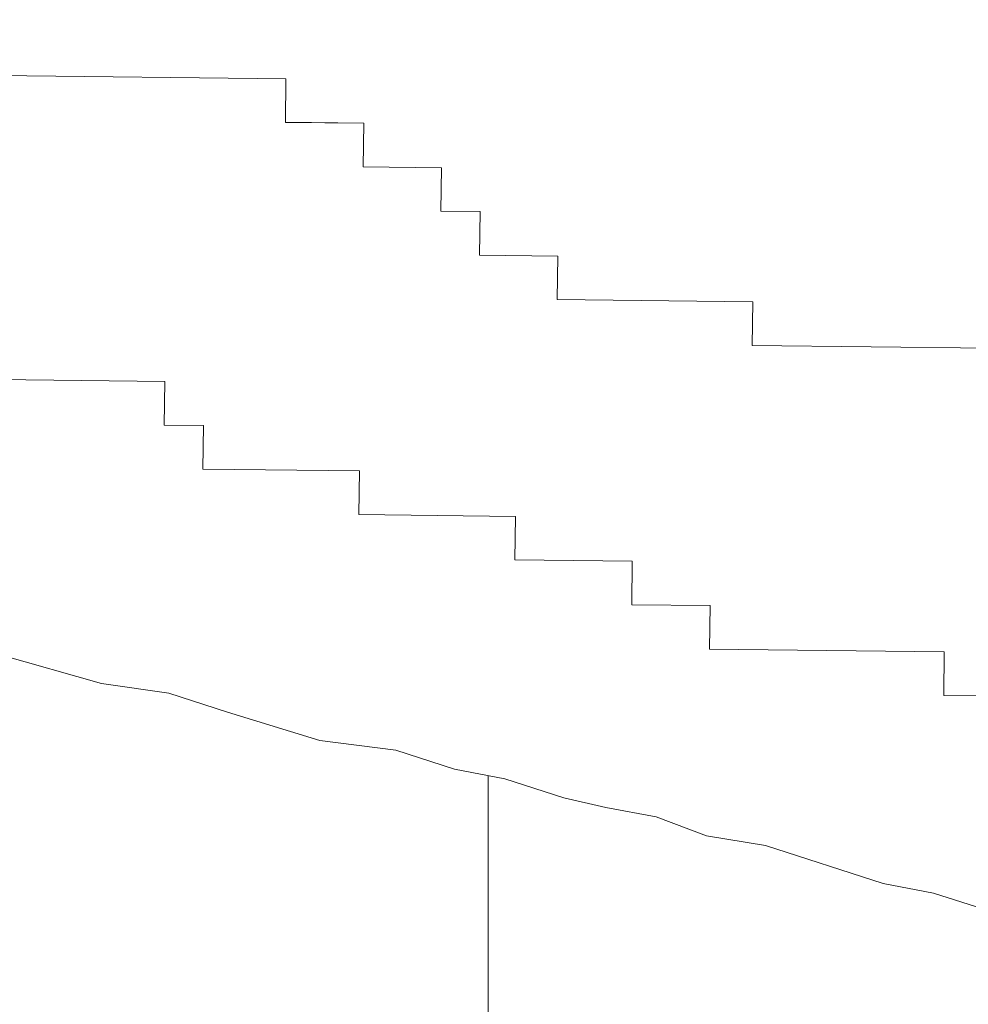
# Model space of a CAD drawing. Units: inches. Extents: x -466983 to 1020, y 324 to 318697.
# Tile 55 of 97: x 634.844 to 637.858, y 939.565 to 942.694. Entities that reach past the tile are written whole.
import ezdxf

# ---------------------------------------------------------------- set-up
doc = ezdxf.new("R2010")
doc.units = ezdxf.units.IN
doc.header["$MEASUREMENT"] = 0
doc.layers.add('A-FLOR-PATT', color=252, linetype='Continuous', lineweight=13)
doc.layers.add('A-FURN', color=8, linetype='Continuous', lineweight=18)

# ---------------------------------------------------------------- blocks, each defined once
blk = doc.blocks.new('L Shaped Sofa')
at = {"ltscale": 2}
for p, q in [((2432.347, 748.1215), (2432.347, 765.179)), ((2429.4248, 748.9121), (2429.7657, 748.8021)), ((2429.7657, 748.8021), (2430.0581, 748.7465)), ((2430.0581, 748.7465), (2430.74, 748.5264)), ((2430.74, 748.5264), (2431.0812, 748.4706)), ((2431.0812, 748.4706), (2431.3733, 748.3608)), ((2431.3733, 748.3608), (2431.6657, 748.3052)), ((2431.6657, 748.3052), (2431.9094, 748.2499)), ((2431.9094, 748.2499), (2432.2503, 748.1398)), ((2432.2503, 748.1398), (2432.5427, 748.0842)), ((2432.5427, 748.0842), (2432.8836, 747.9742)), ((2432.8836, 747.9742), (2433.3224, 747.9179)), ((2433.3224, 747.9179), (2433.8582, 747.7528)), ((2433.8582, 747.7528), (2434.1991, 747.6427)), ((2427.8919, 747.6787), (2429.7066, 747.6565)), ((2429.7066, 747.6565), (2429.7036, 747.4046)), ((2434.1991, 747.6427), (2434.5891, 747.5867)), ((2434.5891, 747.5867), (2435.1737, 747.4213)), ((2429.7036, 747.4046), (2431.0646, 747.388)), ((2431.0646, 747.388), (2431.0615, 747.1361)), ((2431.0615, 747.1361), (2431.5152, 747.1305)), ((2431.5152, 747.1305), (2431.5121, 746.8786)), ((2431.5121, 746.8786), (2432.1926, 746.8703)), ((2432.1926, 746.8703), (2432.1895, 746.6184)), ((2432.1895, 746.6184), (2433.0969, 746.6073)), ((2433.0969, 746.6073), (2433.0938, 746.3554)), ((2433.0938, 746.3554), (2434.0011, 746.3443)), ((2434.0011, 746.3443), (2433.9981, 746.0924)), ((2433.9981, 746.0924), (2434.2249, 746.0896)), ((2434.2249, 746.0896), (2434.2218, 745.8377)), ((2434.2218, 745.8377), (2436.2633, 745.8128)), ((2428.5478, 745.6551), (2430.8162, 745.6274)), ((2430.8162, 745.6274), (2430.8131, 745.3755)), ((2430.8131, 745.3755), (2431.9473, 745.3616)), ((2431.9473, 745.3616), (2431.9442, 745.1097)), ((2431.9442, 745.1097), (2432.3979, 745.1042)), ((2432.3979, 745.1042), (2432.3948, 744.8522)), ((2432.3948, 744.8522), (2432.6216, 744.8495)), ((2432.6216, 744.8495), (2432.6186, 744.5976)), ((2432.6186, 744.5976), (2433.0722, 744.592)), ((2433.0722, 744.592), (2433.0692, 744.3401)), ((2433.0692, 744.3401), (2433.5228, 744.3346)), ((2433.5228, 744.3346), (2433.5198, 744.0827)), ((2433.5198, 744.0827), (2436.015, 744.0522))]:
    blk.add_line(p, q, dxfattribs=at)

msp = doc.modelspace()

# ---------------------------------------------------------------- hatches: boundary and pattern name
at = {"layer": 'A-FLOR-PATT', "transparency": 33554572}
h = msp.add_hatch(dxfattribs=at)
h.set_pattern_fill('ANSI37', color=256, scale=30)
h.set_pattern_definition([(45, (-1212.4137, -290.035), (-2.6516504, 2.6516504), []), (135, (-1212.4137, -290.035), (-2.6516504, -2.6516504), [])])
h.paths.add_polyline_path([(901.8057, 1075.9377), (900.6144, 1075.9377), (900.6144, 1065.3856), (899.391, 1065.3856), (898.0911, 1065.3856), (892.8356, 1058.7098, -0.258377), (892.1875, 1058.3509), (879.9848, 1058.3509, -0.20177), (879.4382, 1058.5808), (874.0812, 1065.3856), (872.7813, 1065.3856), (871.5579, 1065.3856), (871.5579, 1075.9377), (813.8057, 1075.9377), (813.8057, 1044.7922), (832.3947, 1044.7922, -0.394795), (848.6602, 1028.5356), (848.6602, 1009.9377), (901.8057, 1009.9377), (901.8057, 1015.9377), (901.3057, 1015.9377), (871.3057, 1015.9377), (871.3057, 1017.2502), (871.3344, 1017.2502, -0.401453), (901.3057, 1045.9377), (901.8057, 1045.9377)])
edge = h.paths.add_edge_path(flags=16)
edge.add_line((847.7731, 1068.9486), (847.7731, 1073.7088))
edge.add_arc((849.2269, 1073.7088), 1.4538, 90, 180, ccw=False)
edge.add_line((849.2269, 1075.1627), (864.4921, 1075.1627))
edge.add_arc((864.4921, 1073.7088), 1.4538, 0, 90, ccw=False)
edge.add_line((865.9459, 1073.7088), (865.9459, 1069.0035))
edge.add_arc((832.6447, 1068.9761), 33.3012, -20.61234, 0.04725, ccw=False)
edge.add_ellipse((856.8595, 1058.48), major_axis=(0, 10.2131), ratio=0.6859192, start_angle=100.00884, end_angle=259.99116, ccw=False)
edge.add_arc((881.0742, 1068.9761), 33.3012, 180.04725, 200.61234, ccw=False)
h.paths.add_polyline_path([(853.1456, 1066.4815), (853.1456, 1066.4534), (853.1463, 1066.4534, 0.433107), (852.9166, 1066.6849), (852.9166, 1066.4534), (853.1456, 1066.4534), (853.1456, 1066.4815), (853.088, 1066.6122, 0.697939), (852.6995, 1066.4534), (852.7003, 1066.4534), (852.7003, 1066.4815), (852.9166, 1067.0012), (852.9166, 1066.6849, -0.396254)], flags=0)
h.paths.add_polyline_path([(861.0187, 1066.4815), (861.0187, 1066.4534), (861.0194, 1066.4534, 0.416404), (860.8024, 1066.6849), (860.8024, 1066.4534), (861.0187, 1066.4534), (861.0187, 1066.4815), (860.9672, 1066.6053, 0.713344), (860.5726, 1066.4534), (860.5734, 1066.4534), (860.5734, 1066.4815), (860.8024, 1067.0012), (860.8024, 1066.6849, -0.379973)], flags=0)
edge = h.paths.add_edge_path(flags=0)
edge.add_spline(control_points=[(861.1298, 1065.7855), (861.4661, 1065.2478), (861.6134, 1065.0161), (861.9833, 1064.3736), (862.1924, 1063.9443), (862.5614, 1063.0391), (862.7212, 1062.5633), (862.9865, 1061.5781), (863.092, 1061.0689), (863.2452, 1060.031), (863.293, 1059.5025), (863.3295, 1058.4409), (863.3181, 1057.9078), (863.2366, 1056.8518), (863.1664, 1056.3289), (862.9695, 1055.308), (862.8427, 1054.8099), (862.5365, 1053.8522), (862.3571, 1053.3927), (861.9514, 1052.5249), (861.7251, 1052.1166), (861.233, 1051.3622), (860.9672, 1051.0162), (860.4048, 1050.3949), (860.1082, 1050.1197), (859.4937, 1049.6461), (859.1758, 1049.4476), (858.5276, 1049.1299), (858.1973, 1049.0107), (857.5315, 1048.8518), (857.1959, 1048.8121), (856.5249, 1048.812), (856.1894, 1048.8515), (855.5236, 1049.0101), (855.1933, 1049.1291), (854.545, 1049.4465), (854.2271, 1049.6449), (853.6124, 1050.1183), (853.3158, 1050.3933), (852.7533, 1051.0143), (852.4874, 1051.3602), (851.9952, 1052.1144), (851.7688, 1052.5225), (851.3629, 1053.3902), (851.1834, 1053.8496), (850.877, 1054.8071), (850.7501, 1055.3051), (850.553, 1056.326), (850.4827, 1056.8488), (850.401, 1057.9048), (850.3895, 1058.4379), (850.4257, 1059.4995), (850.4734, 1060.0281), (850.6265, 1061.066), (850.7318, 1061.5753), (850.9969, 1062.5605), (851.1567, 1063.0365), (851.5254, 1063.9418), (851.7345, 1064.3712), (852.1056, 1065.0164), (852.2544, 1065.2503), (852.6082, 1065.7335)], knot_values=[3.915332, 3.915332, 3.915332, 3.915332, 4.013468, 4.013468, 4.175532, 4.175532, 4.337596, 4.337596, 4.49966, 4.49966, 4.661724, 4.661724, 4.823788, 4.823788, 4.985852, 4.985852, 5.147916, 5.147916, 5.30998, 5.30998, 5.472044, 5.472044, 5.634109, 5.634109, 5.796173, 5.796173, 5.958237, 5.958237, 6.120301, 6.120301, 6.282365, 6.282365, 6.444429, 6.444429, 6.606493, 6.606493, 6.768557, 6.768557, 6.930621, 6.930621, 7.092685, 7.092685, 7.254749, 7.254749, 7.416813, 7.416813, 7.578878, 7.578878, 7.740942, 7.740942, 7.903006, 7.903006, 8.06507, 8.06507, 8.227134, 8.227134, 8.389198, 8.389198, 8.551262, 8.551262, 8.65037, 8.65037, 8.65037, 8.65037], degree=3, periodic=0)
edge.add_line((852.6421, 1065.7855), (861.1298, 1065.7855))
edge = h.paths.add_edge_path(flags=0)
edge.add_ellipse((856.8496, 1057.7432), major_axis=(0, 7.7921), ratio=0.687861, start_angle=0, end_angle=360)
h.paths.add_polyline_path([(848.8634, 1069.3891), (848.8634, 1073.9605, -0.414214), (849.9538, 1075.0508), (863.7652, 1075.0508, -0.414214), (864.8555, 1073.9605), (864.8555, 1069.3891, -0.388936), (864.5237, 1069.027, -0.043561), (849.1953, 1069.027, -0.388936)], flags=0)
h.paths.add_polyline_path([(853.1006, 1068.1122, -1), (852.6775, 1068.1122, -1)], flags=0)
edge = h.paths.add_edge_path(flags=0)
edge.add_ellipse((856.8595, 1057.3378), major_axis=(0, 2.207), ratio=0.657164, start_angle=0, end_angle=360)
h.paths.add_polyline_path([(861.0415, 1068.1122, -1), (860.6184, 1068.1122, -1)], flags=0)
edge = h.paths.add_edge_path()
edge.add_line((573.9537, 1057.3412), (573.9537, 1075.9377))
edge.add_line((573.9537, 1075.9377), (558.7308, 1075.9377))
edge.add_line((558.7308, 1075.9377), (558.7308, 1065.3856))
edge.add_line((558.7308, 1065.3856), (557.5074, 1065.3856))
edge.add_line((557.5074, 1065.3856), (556.2075, 1065.3856))
edge.add_line((556.2075, 1065.3856), (550.952, 1058.7098))
edge.add_arc((550.3039, 1059.1155), 0.7646, 270, 327.9483, ccw=False)
edge.add_line((550.3039, 1058.3509), (538.1012, 1058.3509))
edge.add_arc((538.1012, 1059.1155), 0.7646, 224.3704, 270, ccw=False)
edge.add_line((537.5546, 1058.5808), (532.1976, 1065.3856))
edge.add_line((532.1976, 1065.3856), (530.8977, 1065.3856))
edge.add_line((530.8977, 1065.3856), (529.6743, 1065.3856))
edge.add_line((529.6743, 1065.3856), (529.6743, 1075.9377))
edge.add_line((529.6743, 1075.9377), (520.8057, 1075.9377))
edge.add_line((520.8057, 1075.9377), (520.8057, 1045.9377))
edge.add_line((520.8057, 1045.9377), (521.3057, 1045.9377))
edge.add_arc((521.3057, 1015.9377), 30, 2.50749, 90, ccw=False)
edge.add_line((551.277, 1017.2502), (551.3057, 1017.2502))
edge.add_line((551.3057, 1017.2502), (551.3057, 1015.9377))
edge.add_line((551.3057, 1015.9377), (520.8057, 1015.9377))
edge.add_line((520.8057, 1015.9377), (520.8057, 1009.9377))
edge.add_line((520.8057, 1009.9377), (559.1913, 1010.4022))
edge.add_arc((559.1913, 1011.856), 1.4538, 180, 270, ccw=False)
edge.add_line((557.7375, 1011.856), (557.7375, 1016.5613))
edge.add_arc((591.0386, 1016.5888), 33.3012, 159.38766, 180.04725, ccw=False)
edge.add_ellipse((566.8239, 1027.0848), major_axis=(0, 10.2131), ratio=0.6859192, start_angle=280.00884, end_angle=439.99116, ccw=False)
edge.add_arc((542.6091, 1016.5888), 33.3012, 0.04725, 20.61234, ccw=False)
edge.add_line((575.9103, 1016.6162), (575.9103, 1011.856))
edge.add_arc((574.4565, 1011.856), 1.4538, -90, 0, ccw=False)
edge.add_line((574.4565, 1010.4022), (608.8057, 1009.9377))
edge.add_line((608.8057, 1009.9377), (608.8057, 1041.0857))
edge.add_line((608.8057, 1041.0857), (590.2179, 1041.0857))
edge.add_arc((590.775, 1057.9074), 16.8309, 181.92775, 268.10321, ccw=False)
edge = h.paths.add_edge_path()
edge.add_ellipse((494.2443, 583.6204), major_axis=(0, 10.2131), ratio=0.6859192, start_angle=280.00884, end_angle=439.99116, ccw=False)
edge.add_arc((470.0296, 573.1243), 33.3012, 0.04725, 20.61234, ccw=False)
edge.add_line((503.3307, 573.1518), (503.3307, 568.3916))
edge.add_arc((501.8769, 568.3916), 1.4538, -90, 0, ccw=False)
edge.add_line((501.8769, 566.9377), (539.8057, 566.9377))
edge.add_line((539.8057, 566.9377), (539.8057, 572.9377))
edge.add_line((539.8057, 572.9377), (539.3057, 572.9377))
edge.add_line((539.3057, 572.9377), (509.3057, 572.9377))
edge.add_line((509.3057, 572.9377), (509.3057, 574.2502))
edge.add_line((509.3057, 574.2502), (509.3344, 574.2502))
edge.add_arc((539.3057, 572.9377), 30, 90, 177.49251, ccw=False)
edge.add_line((539.3057, 602.9377), (539.8057, 602.9377))
edge.add_line((539.8057, 602.9377), (539.8057, 626.9377))
edge.add_line((539.8057, 626.9377), (531.7718, 626.9377))
edge.add_line((531.7718, 626.9377), (531.7718, 616.3856))
edge.add_line((531.7718, 616.3856), (530.5484, 616.3856))
edge.add_line((530.5484, 616.3856), (529.2485, 616.3856))
edge.add_line((529.2485, 616.3856), (523.7105, 609.3509))
edge.add_line((523.7105, 609.3509), (510.7766, 609.3509))
edge.add_line((510.7766, 609.3509), (505.2386, 616.3856))
edge.add_line((505.2386, 616.3856), (503.9387, 616.3856))
edge.add_line((503.9387, 616.3856), (502.7153, 616.3856))
edge.add_line((502.7153, 616.3856), (502.7153, 626.9377))
edge.add_line((502.7153, 626.9377), (481.6983, 626.9377))
edge.add_line((481.6983, 626.9377), (481.6983, 610.995))
edge.add_arc((467.2703, 611.4728), 14.4359, 271.92775, 358.10321, ccw=False)
edge.add_line((467.7559, 597.0451), (451.8057, 597.0451))
edge.add_line((451.8057, 597.0451), (451.8057, 584.4035))
edge.add_line((451.8057, 584.4035), (451.8057, 566.9377))
edge.add_line((451.8057, 566.9377), (486.6117, 566.9377))
edge.add_arc((486.6117, 568.3916), 1.4538, 180, 270, ccw=False)
edge.add_line((485.1579, 568.3916), (485.1579, 573.0969))
edge.add_arc((518.4591, 573.1243), 33.3012, 159.38766, 180.04725, ccw=False)
h.paths.add_polyline_path([(836.2609, 1020.7328), (879.8898, 1020.7328), (879.8898, 1039.3902), (836.2609, 1039.3902)], flags=25)
h.paths.add_polyline_path([(549.9851, 1036.7492), (593.614, 1036.7492), (593.614, 1055.4065), (549.9851, 1055.4065)], flags=24)
h.paths.add_polyline_path([(475.123, 595.5959), (518.752, 595.5959), (518.752, 614.2532), (475.123, 614.2532)], flags=24)
h = msp.add_hatch(dxfattribs=at)
h.set_pattern_fill('ANSI37', color=256, scale=20)
h.set_pattern_definition([(45, (-1212.4137, -290.035), (-1.767767, 1.767767), []), (135, (-1212.4137, -290.035), (-1.767767, -1.767767), [])])
h.paths.add_polyline_path([(809.8057, 870.9377), (809.8057, 888.1519), (806.9985, 888.1519), (802.6624, 888.1519), (789.3832, 888.1519), (786.2846, 888.1519, -0.414214), (785.4991, 888.9374), (785.4991, 900.1959), (785.4991, 908.4696, -0.414214), (786.8082, 909.7787, -0.414214), (785.4991, 911.0878), (785.4991, 929.1015, -0.414214), (786.8082, 930.4106, -0.414214), (785.4991, 931.7197), (785.4991, 931.9039, -0.414214), (784.19, 930.5948), (766.7223, 930.5948, -0.412359), (765.4132, 931.8956, -0.413741), (764.1145, 930.5782), (744.5781, 930.422, -0.416556), (743.7864, 931.2075), (743.7864, 933.5153), (742.2154, 933.5153), (742.2154, 952.024, -0.001344), (743.7864, 952.1998), (743.7864, 953.9377), (678.5915, 953.9377), (678.5915, 951.1305), (678.5915, 946.7945), (678.5915, 933.5153), (678.5915, 930.4166, -0.414214), (677.806, 929.6312), (666.5475, 929.6312), (658.2738, 929.6312, -0.414214), (656.9647, 930.9403, -0.414214), (655.6556, 929.6312), (637.6419, 929.6312, -0.414214), (636.3328, 930.9403, -0.414214), (635.0237, 929.6312), (634.8395, 929.6312, -0.414214), (636.1486, 928.322), (636.1486, 910.8544, -0.412359), (634.8478, 909.5452, -0.413741), (636.1653, 908.2466), (636.3214, 888.7102, -0.416556), (635.5359, 887.9184), (633.2281, 887.9184), (633.2281, 886.3475), (614.7194, 886.3475, -0.001344), (614.5436, 887.9184), (612.8057, 887.9184), (612.8057, 834.9377), (612.8057, 752.9377), (612.8057, 748.9377), (612.8057, 697.9377), (654.8057, 697.9377), (654.8057, 701.9377), (715.8057, 701.9377), (715.8057, 737.4353), (774.2918, 737.4353), (774.2918, 795.9377), (809.8057, 795.9377)])
h.paths.add_polyline_path([(679.2761, 849.5757, 0.102523), (682.1475, 849.2608, -0.080461), (694.5428, 849.7725, -0.283899), (694.4822, 849.0082, 0.136605), (694.4068, 848.8103, -0.030441), (694.5428, 846.8929), (694.5428, 842.6198), (694.5428, 838.3466, -0.028219), (694.4246, 836.5684), (694.425, 836.5684, 0.196187), (694.4456, 836.2708, -0.302897), (694.5428, 835.467, -0.080461), (682.1475, 835.9787, 0.102523), (679.2761, 835.6638, -0.58611), (678.6457, 836.0169), (678.6457, 849.2227, -0.58611)], flags=16)
h.paths.add_polyline_path([(679.5173, 848.6515, 0.699597), (679.476, 848.6342, 1.20716), (679.1935, 848.7422, 0.010621)], flags=0)
h.paths.add_polyline_path([(679.4923, 836.5608, -0.013798), (679.9178, 836.6594, -0.071703), (682.8533, 837.1434, -0.165743), (682.1665, 839.1006), (682.1665, 842.6094), (682.1665, 846.0603, -0.240616), (683.4733, 848.6767, -0.068263), (693.9295, 849.0082), (693.7875, 848.7083), (693.7875, 849.0228, 0.067332), (683.4733, 848.6767, 0.240616), (682.1665, 846.0603), (682.1665, 842.6094), (682.1665, 839.1006, 0.23459), (683.461, 836.5513, 0.068093), (693.7875, 836.1955), (693.7875, 836.5104), (693.9296, 836.2102, -0.077215), (682.2421, 836.7815, 0.086627), (679.5283, 836.5701, -0.628402), (679.5029, 836.5735), (679.5029, 836.6071, 0.910458)], flags=0)
h.paths.add_polyline_path([(679.476, 848.6364), (679.2069, 848.647), (679.2069, 836.5718, 0.913566), (679.3645, 836.5861), (679.476, 836.5824)], flags=0)
h.paths.add_polyline_path([(679.2761, 829.8604, 0.102523), (682.1475, 829.5455, -0.080461), (694.5428, 830.0572, -0.283899), (694.4822, 829.2929, 0.136605), (694.4068, 829.095, -0.030441), (694.5428, 827.1776), (694.5428, 822.9045), (694.5428, 818.6314, -0.028219), (694.4246, 816.8531), (694.425, 816.8532, 0.196187), (694.4456, 816.5555, -0.302897), (694.5428, 815.7517, -0.080461), (682.1475, 816.2635, 0.102523), (679.2761, 815.9485, -0.58611), (678.6457, 816.3016), (678.6457, 829.5074, -0.58611)], flags=16)
h.paths.add_polyline_path([(679.5173, 828.9362, 0.699597), (679.476, 828.9189, 1.20716), (679.1935, 829.0269, 0.010621)], flags=0)
h.paths.add_polyline_path([(679.4923, 816.8456, -0.013798), (679.9178, 816.9441, -0.071703), (682.8533, 817.4281, -0.165743), (682.1665, 819.3853), (682.1665, 822.8941), (682.1665, 826.345, -0.240616), (683.4733, 828.9614, -0.068263), (693.9295, 829.2929), (693.7875, 828.9931), (693.7875, 829.3076, 0.067332), (683.4733, 828.9614, 0.240616), (682.1665, 826.345), (682.1665, 822.8941), (682.1665, 819.3853, 0.23459), (683.461, 816.836, 0.068093), (693.7875, 816.4802), (693.7875, 816.7952), (693.9296, 816.4949, -0.077215), (682.2421, 817.0662, 0.086627), (679.5283, 816.8549, -0.628402), (679.5029, 816.8582), (679.5029, 816.8918, 0.910458)], flags=0)
h.paths.add_polyline_path([(679.476, 828.9211), (679.2069, 828.9317), (679.2069, 816.8565, 0.913566), (679.3645, 816.8708), (679.476, 816.8671)], flags=0)
h.paths.add_polyline_path([(679.2761, 810.1451, 0.102523), (682.1475, 809.8302, -0.080461), (694.5428, 810.342, -0.3023), (694.4466, 809.5394, 0.10023), (694.4058, 809.3878, -0.03057), (694.5428, 807.4623), (694.5428, 803.1892), (694.5428, 798.9161, -0.03057), (694.4058, 796.9906, 0.10023), (694.4466, 796.839, -0.3023), (694.5428, 796.0365, -0.080461), (682.1475, 796.5482, 0.102523), (679.2761, 796.2333, -0.58611), (678.6457, 796.5863), (678.6457, 809.7921, -0.58611)], flags=16)
h.paths.add_polyline_path([(679.5173, 809.2417, 0.699597), (679.476, 809.2244, 1.20716), (679.1935, 809.3324, 0.010621)], flags=0)
h.paths.add_polyline_path([(679.4923, 797.151, -0.013798), (679.9178, 797.2496, -0.071703), (682.8533, 797.7336, -0.165743), (682.1665, 799.6908), (682.1665, 803.1996), (682.1665, 806.6505, -0.239349), (683.461, 809.2577, -0.072465), (694.4468, 809.5405, 0.197932), (694.425, 809.2405), (693.7875, 809.2985), (693.7875, 809.6135, 0.068093), (683.461, 809.2577, 0.239349), (682.1665, 806.6505), (682.1665, 803.1996), (682.1665, 799.6908, 0.235854), (683.4733, 797.1323, 0.067332), (693.7875, 796.7861), (693.7875, 797.1006), (694.425, 797.1586, 0.197932), (694.4468, 796.8586, -0.080419), (682.1557, 797.3795, 0.083867), (679.5283, 797.1603, -0.628402), (679.5029, 797.1637), (679.5029, 797.1973, 0.910458)], flags=0)
h.paths.add_polyline_path([(679.2069, 809.2372), (679.2069, 797.162, 0.913566), (679.3645, 797.1763), (679.476, 797.1726), (679.476, 809.2266)], flags=0)
h.paths.add_polyline_path([(695.3643, 853.2989), (728.2231, 853.2989), (728.2231, 771.1519), (695.3643, 771.1519)], flags=16)
h.paths.add_polyline_path([(696.0215, 852.6417), (727.5659, 852.6417), (727.5659, 771.809), (696.0215, 771.809)], flags=0)
h.paths.add_polyline_path([(679.2761, 788.7869, 0.102523), (682.1475, 788.472, -0.080461), (694.5428, 788.9837, -0.3023), (694.4466, 788.1812, 0.10023), (694.4058, 788.0296, -0.03057), (694.5428, 786.1041), (694.5428, 781.831), (694.5428, 777.5578, -0.03057), (694.4058, 775.6323, 0.10023), (694.4466, 775.4808, -0.3023), (694.5428, 774.6782, -0.080461), (682.1475, 775.19, 0.102523), (679.2761, 774.875, -0.58611), (678.6457, 775.2281), (678.6457, 788.4339, -0.58611)], flags=16)
h.paths.add_polyline_path([(679.5173, 787.8834, 0.699597), (679.476, 787.8662, 1.20716), (679.1935, 787.9742, 0.010621)], flags=0)
h.paths.add_polyline_path([(679.4923, 775.7928, -0.013798), (679.9178, 775.8914, -0.071703), (682.8533, 776.3753, -0.165743), (682.1665, 778.3325), (682.1665, 781.8414), (682.1665, 785.2922, -0.239349), (683.461, 787.8995, -0.072465), (694.4468, 788.1823, 0.197932), (694.425, 787.8823), (693.7875, 787.9403), (693.7875, 788.2553, 0.068093), (683.461, 787.8995, 0.239349), (682.1665, 785.2922), (682.1665, 781.8414), (682.1665, 778.3325, 0.235854), (683.4733, 775.7741, 0.067332), (693.7875, 775.4279), (693.7875, 775.7424), (694.425, 775.8004, 0.197932), (694.4468, 775.5004, -0.080419), (682.1557, 776.0212, 0.083867), (679.5283, 775.8021, -0.628402), (679.5029, 775.8054), (679.5029, 775.8391, 0.910458)], flags=0)
h.paths.add_polyline_path([(679.2069, 787.8789), (679.2069, 775.8038, 0.913566), (679.3645, 775.818), (679.476, 775.8144), (679.476, 787.8684)], flags=0)
h.paths.add_polyline_path([(704.641, 854.1204, -0.080461), (705.1527, 866.5157, 0.102523), (704.8378, 869.3871, -0.58611), (705.1908, 870.0174), (718.3966, 870.0174, -0.58611), (718.7496, 869.3871, 0.102523), (718.4347, 866.5157, -0.080461), (718.9465, 854.1204, -0.3023), (718.1439, 854.2166, 0.10023), (717.9924, 854.2574, -0.03057), (716.0668, 854.1204), (711.7937, 854.1204), (707.5206, 854.1204, -0.03057), (705.5951, 854.2574, 0.10023), (705.4435, 854.2166, -0.3023)], flags=16)
h.paths.add_polyline_path([(717.8462, 869.1459, 0.699597), (717.8289, 869.1872, 1.20716), (717.9369, 869.4697, 0.010621)], flags=0)
h.paths.add_polyline_path([(705.4631, 854.2164, -0.080419), (705.984, 866.5074, 0.083867), (705.7648, 869.1349, -0.628402), (705.7682, 869.1603), (705.8018, 869.1603, 0.910458), (705.7555, 869.1709, -0.013798), (705.8541, 868.7454, -0.071703), (706.3381, 865.8099, -0.165743), (708.2953, 866.4967), (711.8041, 866.4967), (715.255, 866.4967, -0.239349), (717.8622, 865.2022, -0.072465), (718.145, 854.2164, 0.197932), (717.845, 854.2382), (717.903, 854.8757), (718.218, 854.8757, 0.068093), (717.8622, 865.2022, 0.239349), (715.255, 866.4967), (711.8041, 866.4967), (708.2953, 866.4967, 0.235854), (705.7368, 865.1898, 0.067332), (705.3906, 854.8757), (705.7051, 854.8757), (705.7631, 854.2382, 0.197932)], flags=16)
h.paths.add_polyline_path([(705.7665, 869.4563, 0.913566), (705.7808, 869.2987), (705.7771, 869.1872), (717.8311, 869.1872), (717.8417, 869.4563)], flags=0)
h.paths.add_polyline_path([(729.0446, 842.6198), (729.0446, 846.8929, -0.03057), (729.1817, 848.8184, 0.10023), (729.1408, 848.9699, -0.3023), (729.0446, 849.7725, -0.080461), (741.4399, 849.2608, 0.102523), (744.3113, 849.5757, -0.58611), (744.9417, 849.2227), (744.9417, 836.0169, -0.58611), (744.3113, 835.6638, 0.102523), (741.4399, 835.9787, -0.080461), (729.0446, 835.467, -0.3023), (729.1408, 836.2696, 0.10023), (729.1817, 836.4211, -0.03057), (729.0446, 838.3466)], flags=16)
h.paths.add_polyline_path([(744.1115, 836.5846, 1.20716), (744.3939, 836.4766, 0.010621), (744.0701, 836.5673, 0.699597)], flags=0)
h.paths.add_polyline_path([(729.1407, 836.2684, 0.197932), (729.1624, 836.5684), (729.7999, 836.5104), (729.7999, 836.1955, 0.068093), (740.1264, 836.5513, 0.239349), (741.4209, 839.1585), (741.4209, 842.6094), (741.4209, 846.1182, 0.235854), (740.1141, 848.6767, 0.067332), (729.7999, 849.0228), (729.7999, 848.7083), (729.1624, 848.6503, 0.197932), (729.1407, 848.9504, -0.080419), (741.4317, 848.4295, 0.083867), (744.0591, 848.6486, -0.628402), (744.0845, 848.6453), (744.0845, 848.6117, 0.910458), (744.0951, 848.6579, -0.013798), (743.6696, 848.5594, -0.071703), (740.7341, 848.0754, -0.165743), (741.4209, 846.1182), (741.4209, 842.6094), (741.4209, 839.1585, -0.239349), (740.1264, 836.5513, -0.072465)], flags=0)
h.paths.add_polyline_path([(729.0446, 830.0572, -0.080461), (741.4399, 829.5455, 0.102523), (744.3113, 829.8604, -0.58611), (744.9417, 829.5074), (744.9417, 816.3016, -0.58611), (744.3113, 815.9485, 0.102523), (741.4399, 816.2635, -0.080461), (729.0446, 815.7517, -0.3023), (729.1408, 816.5543, 0.10023), (729.1817, 816.7058, -0.03057), (729.0446, 818.6314), (729.0446, 822.9045), (729.0446, 827.1776, -0.03057), (729.1817, 829.1031, 0.10023), (729.1408, 829.2547, -0.3023)], flags=16)
h.paths.add_polyline_path([(744.1115, 816.8693, 1.20716), (744.3939, 816.7613, 0.010621), (744.0701, 816.852, 0.699597)], flags=0)
h.paths.add_polyline_path([(729.1407, 829.2351, -0.080419), (741.4317, 828.7142, 0.083867), (744.0591, 828.9334, -0.628402), (744.0845, 828.93), (744.0845, 828.8964, 0.910458), (744.0951, 828.9427, -0.013798), (743.6696, 828.8441, -0.071703), (740.7341, 828.3601, -0.165743), (741.4209, 826.4029), (741.4209, 822.8941), (741.4209, 819.4432, -0.239349), (740.1264, 816.836, -0.072465), (729.1407, 816.5531, 0.197932), (729.1624, 816.8532), (729.7999, 816.7952), (729.7999, 816.4802, 0.068093), (740.1264, 816.836, 0.239349), (741.4209, 819.4432), (741.4209, 822.8941), (741.4209, 826.4029, 0.235854), (740.1141, 828.9614, 0.067332), (729.7999, 829.3076), (729.7999, 828.9931), (729.1624, 828.9351, 0.197932)], flags=16)
h.paths.add_polyline_path([(729.0446, 810.342, -0.080461), (741.4399, 809.8302, 0.102523), (744.3113, 810.1451, -0.58611), (744.9417, 809.7921), (744.9417, 796.5863, -0.58611), (744.3113, 796.2333, 0.102523), (741.4399, 796.5482, -0.080461), (729.0446, 796.0365, -0.283899), (729.1052, 796.8007, 0.136605), (729.1806, 796.9987, -0.030441), (729.0446, 798.9161), (729.0446, 803.1892), (729.0446, 807.4623, -0.028219), (729.1628, 809.2406), (729.1624, 809.2405, 0.196187), (729.1418, 809.5382, -0.302897)], flags=16)
h.paths.add_polyline_path([(744.1115, 797.1748, 1.20716), (744.3939, 797.0668, 0.010621), (744.0701, 797.1575, 0.699597)], flags=0)
h.paths.add_polyline_path([(741.3453, 809.0275, 0.086627), (744.0591, 809.2388, -0.628402), (744.0845, 809.2355), (744.0845, 809.2019, 0.910458), (744.0951, 809.2481, -0.013798), (743.6696, 809.1496, -0.071703), (740.7341, 808.6656, -0.165743), (741.4209, 806.7084), (741.4209, 803.1996), (741.4209, 799.7487, -0.240616), (740.1141, 797.1323, -0.068263), (729.658, 796.8008), (729.7999, 797.1006), (729.7999, 796.7861, 0.067332), (740.1141, 797.1323, 0.240616), (741.4209, 799.7487), (741.4209, 803.1996), (741.4209, 806.7084, 0.23459), (740.1264, 809.2577, 0.068093), (729.7999, 809.6135), (729.7999, 809.2985), (729.6578, 809.5988, -0.077215)], flags=0)
h.paths.add_polyline_path([(704.641, 770.3304, -0.283899), (705.4053, 770.2697, 0.136605), (705.6032, 770.1944, -0.030441), (707.5206, 770.3304), (711.7937, 770.3304), (716.0668, 770.3304, -0.028219), (717.8451, 770.2122), (717.845, 770.2126, 0.196187), (718.1427, 770.2331, -0.302897), (718.9465, 770.3304, -0.080461), (718.4347, 757.9351, 0.102523), (718.7496, 755.0637, -0.58611), (718.3966, 754.4333), (705.1908, 754.4333, -0.58611), (704.8378, 755.0637, 0.102523), (705.1527, 757.9351, -0.080461)], flags=16)
h.paths.add_polyline_path([(705.762, 755.3048, 0.699597), (705.7793, 755.2635, 1.20716), (705.6713, 754.9811, 0.010621)], flags=0)
h.paths.add_polyline_path([(705.4053, 769.717), (705.7051, 769.5751), (705.3906, 769.5751, 0.067332), (705.7368, 759.2609, 0.240616), (708.3532, 757.954), (711.8041, 757.954), (715.3129, 757.954, 0.23459), (717.8622, 759.2485, 0.068093), (718.218, 769.5751), (717.903, 769.5751), (718.2033, 769.7172, -0.077215), (717.632, 758.0297, 0.086627), (717.8433, 755.3159, -0.628402), (717.84, 755.2904), (717.8064, 755.2904, 0.910458), (717.8526, 755.2799, -0.013798), (717.7541, 755.7053, -0.071703), (717.2701, 758.6409, -0.165743), (715.3129, 757.954), (711.8041, 757.954), (708.3532, 757.954, -0.240616), (705.7368, 759.2609, -0.068263)], flags=0)
h.paths.add_polyline_path([(729.0446, 788.9837, -0.080461), (741.4399, 788.472, 0.102523), (744.3113, 788.7869, -0.58611), (744.9417, 788.4339), (744.9417, 775.2281, -0.58611), (744.3113, 774.875, 0.102523), (741.4399, 775.19, -0.080461), (729.0446, 774.6782, -0.283899), (729.1052, 775.4425, 0.136605), (729.1806, 775.6405, -0.030441), (729.0446, 777.5578), (729.0446, 781.831), (729.0446, 786.1041, -0.028219), (729.1628, 787.8823), (729.1624, 787.8823, 0.196187), (729.1418, 788.1799, -0.302897)], flags=16)
h.paths.add_polyline_path([(744.1115, 775.8165, 1.20716), (744.3939, 775.7086, 0.010621), (744.0701, 775.7993, 0.699597)], flags=0)
h.paths.add_polyline_path([(741.3453, 787.6692, 0.086627), (744.0591, 787.8806, -0.628402), (744.0845, 787.8773), (744.0845, 787.8437, 0.910458), (744.0951, 787.8899, -0.013798), (743.6696, 787.7913, -0.071703), (740.7341, 787.3074, -0.165743), (741.4209, 785.3502), (741.4209, 781.8414), (741.4209, 778.3905, -0.240616), (740.1141, 775.7741, -0.068263), (729.658, 775.4425), (729.7999, 775.7424), (729.7999, 775.4279, 0.067332), (740.1141, 775.7741, 0.240616), (741.4209, 778.3905), (741.4209, 781.8414), (741.4209, 785.3502, 0.23459), (740.1264, 787.8995, 0.068093), (729.7999, 788.2553), (729.7999, 787.9403), (729.6578, 788.2405, -0.077215)], flags=0)
h.paths.add_polyline_path([(744.1115, 848.6364), (744.1115, 836.5824), (744.3805, 836.5718), (744.3805, 848.647, 0.913566), (744.2229, 848.6327)], flags=0)
h.paths.add_polyline_path([(744.2229, 828.9174), (744.1115, 828.9211), (744.1115, 816.8671), (744.3805, 816.8565), (744.3805, 828.9317, 0.913566)], flags=0)
h.paths.add_polyline_path([(717.8311, 755.2635), (705.7771, 755.2635), (705.7665, 754.9945), (717.8417, 754.9945, 0.913566), (717.8274, 755.1521)], flags=0)
h.paths.add_polyline_path([(744.2229, 809.2229), (744.1115, 809.2266), (744.1115, 797.1726), (744.3805, 797.162), (744.3805, 809.2372, 0.913566)], flags=0)
h.paths.add_polyline_path([(744.1115, 787.8684), (744.1115, 775.8144), (744.3805, 775.8038), (744.3805, 787.8789, 0.913566), (744.2229, 787.8647)], flags=0)
h.paths.add_polyline_path([(678.8774, 877.1228), (737.6127, 877.1228), (737.6127, 899.5116), (678.8774, 899.5116)], flags=24)

# ---------------------------------------------------------------- linework, layer by layer
at = {"layer": 'A-FURN', "ltscale": 2}
for p, q in [((635.6899, 942.5057), (634.3219, 942.5224)), ((635.6899, 942.5057), (634.3219, 942.5224)), ((635.6899, 942.5057), (634.3219, 942.5224)), ((635.6899, 942.5057), (634.3219, 942.5224)), ((635.6899, 942.5057), (634.3219, 942.5224)), ((635.6899, 942.5057), (634.3219, 942.5224)), ((635.6882, 942.3676), (635.6899, 942.5057)), ((635.6882, 942.3676), (635.6899, 942.5057)), ((635.6882, 942.3676), (635.6899, 942.5057)), ((635.6882, 942.3676), (635.6899, 942.5057)), ((635.6882, 942.3676), (635.6899, 942.5057)), ((635.6882, 942.3676), (635.6899, 942.5057)), ((635.9369, 942.3645), (635.6882, 942.3676)), ((635.9369, 942.3645), (635.6882, 942.3676)), ((635.9369, 942.3645), (635.6882, 942.3676)), ((635.9369, 942.3645), (635.6882, 942.3676)), ((635.9369, 942.3645), (635.6882, 942.3676)), ((635.9369, 942.3645), (635.6882, 942.3676)), ((635.9352, 942.2264), (635.9369, 942.3645)), ((635.9352, 942.2264), (635.9369, 942.3645)), ((635.9352, 942.2264), (635.9369, 942.3645)), ((635.9352, 942.2264), (635.9369, 942.3645)), ((635.9352, 942.2264), (635.9369, 942.3645)), ((635.9352, 942.2264), (635.9369, 942.3645)), ((636.1839, 942.2234), (635.9352, 942.2264)), ((636.1839, 942.2234), (635.9352, 942.2264)), ((636.1839, 942.2234), (635.9352, 942.2264)), ((636.1839, 942.2234), (635.9352, 942.2264)), ((636.1839, 942.2234), (635.9352, 942.2264)), ((636.1839, 942.2234), (635.9352, 942.2264)), ((636.1822, 942.0853), (636.1839, 942.2234)), ((636.1822, 942.0853), (636.1839, 942.2234)), ((636.1822, 942.0853), (636.1839, 942.2234)), ((636.1822, 942.0853), (636.1839, 942.2234)), ((636.1822, 942.0853), (636.1839, 942.2234)), ((636.1822, 942.0853), (636.1839, 942.2234)), ((636.3066, 942.0838), (636.1822, 942.0853)), ((636.3066, 942.0838), (636.1822, 942.0853)), ((636.3066, 942.0838), (636.1822, 942.0853)), ((636.3066, 942.0838), (636.1822, 942.0853)), ((636.3066, 942.0838), (636.1822, 942.0853)), ((636.3066, 942.0838), (636.1822, 942.0853)), ((636.3049, 941.9457), (636.3066, 942.0838)), ((636.3049, 941.9457), (636.3066, 942.0838)), ((636.3049, 941.9457), (636.3066, 942.0838)), ((636.3049, 941.9457), (636.3066, 942.0838)), ((636.3049, 941.9457), (636.3066, 942.0838)), ((636.3049, 941.9457), (636.3066, 942.0838)), ((636.5536, 941.9426), (636.3049, 941.9457)), ((636.5536, 941.9426), (636.3049, 941.9457)), ((636.5536, 941.9426), (636.3049, 941.9457)), ((636.5536, 941.9426), (636.3049, 941.9457)), ((636.5536, 941.9426), (636.3049, 941.9457)), ((636.5536, 941.9426), (636.3049, 941.9457)), ((636.5519, 941.8045), (636.5536, 941.9426)), ((636.5519, 941.8045), (636.5536, 941.9426)), ((636.5519, 941.8045), (636.5536, 941.9426)), ((636.5519, 941.8045), (636.5536, 941.9426)), ((636.5519, 941.8045), (636.5536, 941.9426)), ((636.5519, 941.8045), (636.5536, 941.9426)), ((637.1737, 941.7969), (636.5519, 941.8045)), ((637.1737, 941.7969), (636.5519, 941.8045)), ((637.1737, 941.7969), (636.5519, 941.8045)), ((637.1737, 941.7969), (636.5519, 941.8045)), ((637.1737, 941.7969), (636.5519, 941.8045)), ((637.1737, 941.7969), (636.5519, 941.8045)), ((637.172, 941.6588), (637.1737, 941.7969)), ((637.172, 941.6588), (637.1737, 941.7969)), ((637.172, 941.6588), (637.1737, 941.7969)), ((637.172, 941.6588), (637.1737, 941.7969)), ((637.172, 941.6588), (637.1737, 941.7969)), ((637.172, 941.6588), (637.1737, 941.7969)), ((638.4155, 941.6436), (637.172, 941.6588)), ((638.4155, 941.6436), (637.172, 941.6588)), ((638.4155, 941.6436), (637.172, 941.6588)), ((638.4155, 941.6436), (637.172, 941.6588)), ((638.4155, 941.6436), (637.172, 941.6588)), ((638.4155, 941.6436), (637.172, 941.6588)), ((635.305, 941.5435), (634.1858, 941.5572)), ((635.305, 941.5435), (634.1858, 941.5572)), ((635.305, 941.5435), (634.1858, 941.5572)), ((635.305, 941.5435), (634.1858, 941.5572)), ((635.305, 941.5435), (634.1858, 941.5572)), ((635.305, 941.5435), (634.1858, 941.5572)), ((635.3033, 941.4054), (635.305, 941.5435)), ((635.3033, 941.4054), (635.305, 941.5435)), ((635.3033, 941.4054), (635.305, 941.5435)), ((635.3033, 941.4054), (635.305, 941.5435)), ((635.3033, 941.4054), (635.305, 941.5435)), ((635.3033, 941.4054), (635.305, 941.5435)), ((635.4276, 941.4039), (635.3033, 941.4054)), ((635.4276, 941.4039), (635.3033, 941.4054)), ((635.4276, 941.4039), (635.3033, 941.4054)), ((635.4276, 941.4039), (635.3033, 941.4054)), ((635.4276, 941.4039), (635.3033, 941.4054)), ((635.4276, 941.4039), (635.3033, 941.4054)), ((635.426, 941.2658), (635.4276, 941.4039)), ((635.426, 941.2658), (635.4276, 941.4039)), ((635.426, 941.2658), (635.4276, 941.4039)), ((635.426, 941.2658), (635.4276, 941.4039)), ((635.426, 941.2658), (635.4276, 941.4039)), ((635.426, 941.2658), (635.4276, 941.4039)), ((635.9234, 941.2597), (635.426, 941.2658)), ((635.9234, 941.2597), (635.426, 941.2658)), ((635.9234, 941.2597), (635.426, 941.2658)), ((635.9234, 941.2597), (635.426, 941.2658)), ((635.9234, 941.2597), (635.426, 941.2658)), ((635.9234, 941.2597), (635.426, 941.2658)), ((635.9217, 941.1216), (635.9234, 941.2597)), ((635.9217, 941.1216), (635.9234, 941.2597)), ((635.9217, 941.1216), (635.9234, 941.2597)), ((635.9217, 941.1216), (635.9234, 941.2597)), ((635.9217, 941.1216), (635.9234, 941.2597)), ((635.9217, 941.1216), (635.9234, 941.2597)), ((636.4191, 941.1155), (635.9217, 941.1216)), ((636.4191, 941.1155), (635.9217, 941.1216)), ((636.4191, 941.1155), (635.9217, 941.1216)), ((636.4191, 941.1155), (635.9217, 941.1216)), ((636.4191, 941.1155), (635.9217, 941.1216)), ((636.4191, 941.1155), (635.9217, 941.1216)), ((636.4174, 940.9774), (636.4191, 941.1155)), ((636.4174, 940.9774), (636.4191, 941.1155)), ((636.4174, 940.9774), (636.4191, 941.1155)), ((636.4174, 940.9774), (636.4191, 941.1155)), ((636.4174, 940.9774), (636.4191, 941.1155)), ((636.4174, 940.9774), (636.4191, 941.1155)), ((636.7905, 940.9729), (636.4174, 940.9774)), ((636.7905, 940.9729), (636.4174, 940.9774)), ((636.7905, 940.9729), (636.4174, 940.9774)), ((636.7905, 940.9729), (636.4174, 940.9774)), ((636.7905, 940.9729), (636.4174, 940.9774)), ((636.7905, 940.9729), (636.4174, 940.9774)), ((636.7888, 940.8348), (636.7905, 940.9729)), ((636.7888, 940.8348), (636.7905, 940.9729)), ((636.7888, 940.8348), (636.7905, 940.9729)), ((636.7888, 940.8348), (636.7905, 940.9729)), ((636.7888, 940.8348), (636.7905, 940.9729)), ((636.7888, 940.8348), (636.7905, 940.9729)), ((637.0375, 940.8317), (636.7888, 940.8348)), ((637.0375, 940.8317), (636.7888, 940.8348)), ((637.0375, 940.8317), (636.7888, 940.8348)), ((637.0375, 940.8317), (636.7888, 940.8348)), ((637.0375, 940.8317), (636.7888, 940.8348)), ((637.0375, 940.8317), (636.7888, 940.8348)), ((637.0358, 940.6936), (637.0375, 940.8317)), ((637.0358, 940.6936), (637.0375, 940.8317)), ((637.0358, 940.6936), (637.0375, 940.8317)), ((637.0358, 940.6936), (637.0375, 940.8317)), ((637.0358, 940.6936), (637.0375, 940.8317)), ((637.0358, 940.6936), (637.0375, 940.8317)), ((635.1036, 940.5847), (634.7832, 940.6754)), ((635.1036, 940.5847), (634.7832, 940.6754)), ((635.1036, 940.5847), (634.7832, 940.6754)), ((635.1036, 940.5847), (634.7832, 940.6754)), ((635.1036, 940.5847), (634.7832, 940.6754)), ((635.1036, 940.5847), (634.7832, 940.6754)), ((637.782, 940.6845), (637.0358, 940.6936)), ((637.782, 940.6845), (637.0358, 940.6936)), ((637.782, 940.6845), (637.0358, 940.6936)), ((637.782, 940.6845), (637.0358, 940.6936)), ((637.782, 940.6845), (637.0358, 940.6936)), ((637.782, 940.6845), (637.0358, 940.6936)), ((637.7803, 940.5464), (637.782, 940.6845)), ((637.7803, 940.5464), (637.782, 940.6845)), ((637.7803, 940.5464), (637.782, 940.6845)), ((637.7803, 940.5464), (637.782, 940.6845)), ((637.7803, 940.5464), (637.782, 940.6845)), ((637.7803, 940.5464), (637.782, 940.6845)), ((635.3174, 940.554), (635.1036, 940.5847)), ((635.3174, 940.554), (635.1036, 940.5847)), ((635.3174, 940.554), (635.1036, 940.5847)), ((635.3174, 940.554), (635.1036, 940.5847)), ((635.3174, 940.554), (635.1036, 940.5847)), ((635.3174, 940.554), (635.1036, 940.5847)), ((635.5043, 940.4937), (635.3174, 940.554)), ((635.5043, 940.4937), (635.3174, 940.554)), ((635.5043, 940.4937), (635.3174, 940.554)), ((635.5043, 940.4937), (635.3174, 940.554)), ((635.5043, 940.4937), (635.3174, 940.554)), ((635.5043, 940.4937), (635.3174, 940.554)), ((638.7751, 940.5343), (637.7803, 940.5464)), ((638.7751, 940.5343), (637.7803, 940.5464)), ((638.7751, 940.5343), (637.7803, 940.5464)), ((638.7751, 940.5343), (637.7803, 940.5464)), ((638.7751, 940.5343), (637.7803, 940.5464)), ((638.7751, 940.5343), (637.7803, 940.5464)), ((635.798, 940.4031), (635.5043, 940.4937)), ((635.798, 940.4031), (635.5043, 940.4937)), ((635.798, 940.4031), (635.5043, 940.4937)), ((635.798, 940.4031), (635.5043, 940.4937)), ((635.798, 940.4031), (635.5043, 940.4937)), ((635.798, 940.4031), (635.5043, 940.4937)), ((636.0386, 940.3723), (635.798, 940.4031)), ((636.0386, 940.3723), (635.798, 940.4031)), ((636.0386, 940.3723), (635.798, 940.4031)), ((636.0386, 940.3723), (635.798, 940.4031)), ((636.0386, 940.3723), (635.798, 940.4031)), ((636.0386, 940.3723), (635.798, 940.4031)), ((636.2255, 940.3119), (636.0386, 940.3723)), ((636.2255, 940.3119), (636.0386, 940.3723)), ((636.2255, 940.3119), (636.0386, 940.3723)), ((636.2255, 940.3119), (636.0386, 940.3723)), ((636.2255, 940.3119), (636.0386, 940.3723)), ((636.2255, 940.3119), (636.0386, 940.3723)), ((636.3858, 940.2815), (636.2255, 940.3119)), ((636.3858, 940.2815), (636.2255, 940.3119)), ((636.3858, 940.2815), (636.2255, 940.3119)), ((636.3858, 940.2815), (636.2255, 940.3119)), ((636.3858, 940.2815), (636.2255, 940.3119)), ((636.3858, 940.2815), (636.2255, 940.3119)), ((636.3328, 940.2915), (636.3328, 930.9403)), ((636.3328, 940.2915), (636.3328, 930.9403)), ((636.3328, 940.2915), (636.3328, 930.9403)), ((636.3328, 940.2915), (636.3328, 930.9403)), ((636.3328, 940.2915), (636.3328, 930.9403)), ((636.3328, 940.2915), (636.3328, 930.9403)), ((636.5727, 940.2211), (636.3858, 940.2815)), ((636.5727, 940.2211), (636.3858, 940.2815)), ((636.5727, 940.2211), (636.3858, 940.2815)), ((636.5727, 940.2211), (636.3858, 940.2815)), ((636.5727, 940.2211), (636.3858, 940.2815)), ((636.5727, 940.2211), (636.3858, 940.2815)), ((636.7063, 940.1908), (636.5727, 940.2211)), ((636.7063, 940.1908), (636.5727, 940.2211)), ((636.7063, 940.1908), (636.5727, 940.2211)), ((636.7063, 940.1908), (636.5727, 940.2211)), ((636.7063, 940.1908), (636.5727, 940.2211)), ((636.7063, 940.1908), (636.5727, 940.2211)), ((636.8666, 940.1603), (636.7063, 940.1908)), ((636.8666, 940.1603), (636.7063, 940.1908)), ((636.8666, 940.1603), (636.7063, 940.1908)), ((636.8666, 940.1603), (636.7063, 940.1908)), ((636.8666, 940.1603), (636.7063, 940.1908)), ((636.8666, 940.1603), (636.7063, 940.1908)), ((637.0267, 940.1001), (636.8666, 940.1603)), ((637.0267, 940.1001), (636.8666, 940.1603)), ((637.0267, 940.1001), (636.8666, 940.1603)), ((637.0267, 940.1001), (636.8666, 940.1603)), ((637.0267, 940.1001), (636.8666, 940.1603)), ((637.0267, 940.1001), (636.8666, 940.1603)), ((637.2138, 940.0695), (637.0267, 940.1001)), ((637.2138, 940.0695), (637.0267, 940.1001)), ((637.2138, 940.0695), (637.0267, 940.1001)), ((637.2138, 940.0695), (637.0267, 940.1001)), ((637.2138, 940.0695), (637.0267, 940.1001)), ((637.2138, 940.0695), (637.0267, 940.1001)), ((637.5876, 939.9489), (637.2138, 940.0695)), ((637.5876, 939.9489), (637.2138, 940.0695)), ((637.5876, 939.9489), (637.2138, 940.0695)), ((637.5876, 939.9489), (637.2138, 940.0695)), ((637.5876, 939.9489), (637.2138, 940.0695)), ((637.5876, 939.9489), (637.2138, 940.0695)), ((637.7479, 939.9184), (637.5876, 939.9489)), ((637.7479, 939.9184), (637.5876, 939.9489)), ((637.7479, 939.9184), (637.5876, 939.9489)), ((637.7479, 939.9184), (637.5876, 939.9489)), ((637.7479, 939.9184), (637.5876, 939.9489)), ((637.7479, 939.9184), (637.5876, 939.9489)), ((637.9348, 939.8581), (637.7479, 939.9184)), ((637.9348, 939.8581), (637.7479, 939.9184)), ((637.9348, 939.8581), (637.7479, 939.9184)), ((637.9348, 939.8581), (637.7479, 939.9184)), ((637.9348, 939.8581), (637.7479, 939.9184)), ((637.9348, 939.8581), (637.7479, 939.9184))]:
    msp.add_line(p, q, dxfattribs=at)

# ---------------------------------------------------------------- block references
at = {"layer": 'A-FURN', "xscale": 0.5482153745360612, "yscale": 0.5482153745360612, "zscale": 0.5482153745360612, "rotation": 180}
msp.add_blockref('L Shaped Sofa', (1969.7828, 1350.4232), dxfattribs=at)

doc.saveas('drawing.dxf')
